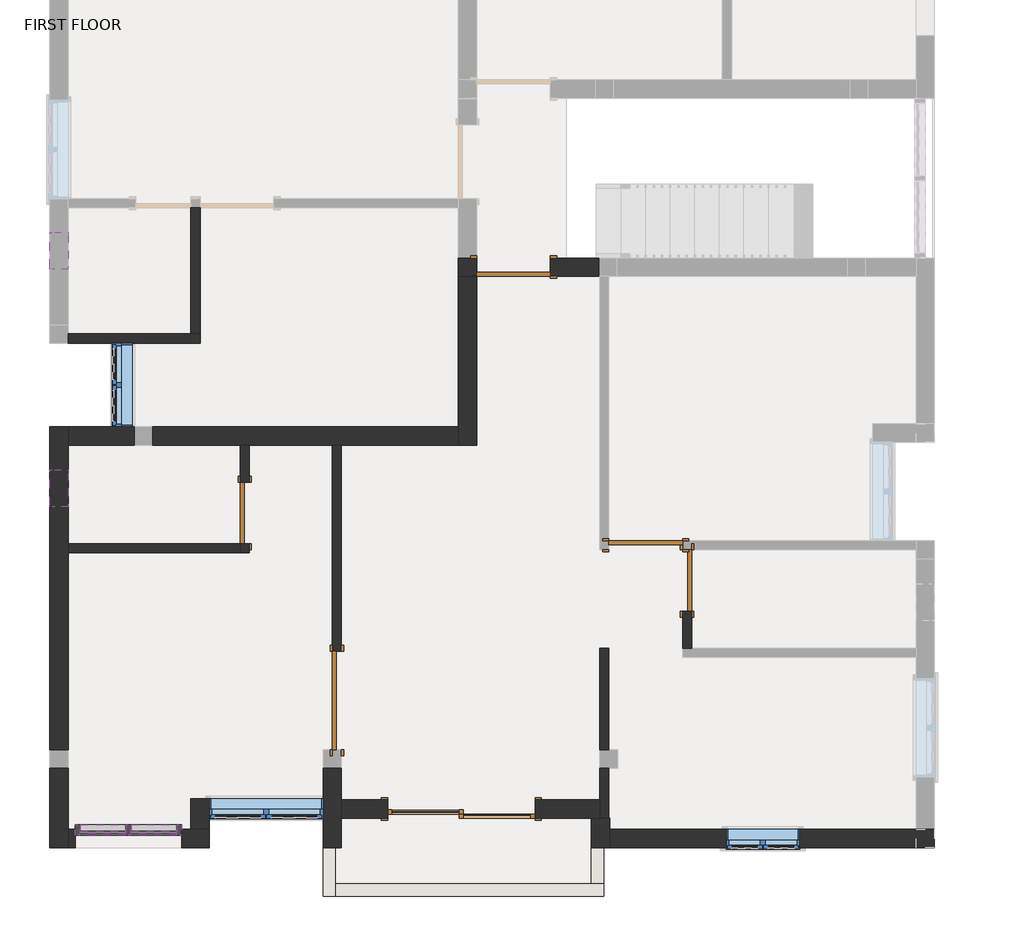
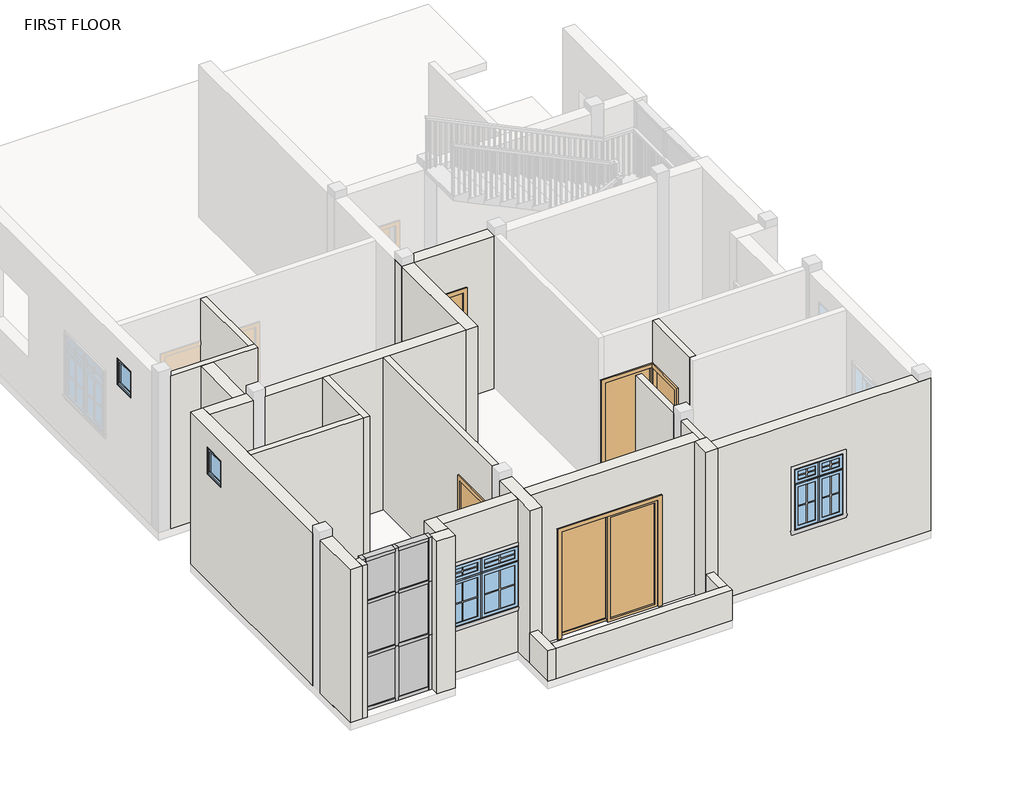
# One storey, part 1 of 6: 25 walls, 17 members, 6 doors, 6 plates, 5 windows.
"""IFC4 building model written with IfcOpenShell, lengths in millimetres."""

from ifc_helpers import new_model, si_unit, frame, origin, place, context, project, spatial, polyline, outline, extrude, faceted_brep, transform, mapped, element, save
from components import door_d4d75d1e, door_78caadf7, single_flush_3_x7_0ca8825f, single_flush_3_x7_305aa2a5, single_flush_4_x7_9343de66, member_6f432376, member_6103f85b, member_e80433b6, member_a715cb85, member_69c8e218, member_c4de40ee, member_049a2e78, member_5cd4c5ac, system_panel_glazed_fbef02e7, system_panel_glazed_b4a8312c, window_abb441dd, window_35f3c129, window_casement_double_awning_double_3_x4_7dc4ce09, window_c5cb33f6

model = new_model("IFC4")

# Units and contexts
model_context = context("Model", 3, world=origin())
ifc_project = project(units=[si_unit("LENGTHUNIT", "METRE", prefix="MILLI")], contexts=[model_context])

# Site, building, storey
site = spatial("IfcSite", under=ifc_project)
building = spatial("IfcBuilding", under=site)
storey = spatial("IfcBuildingStorey", under=building, Name="FIRST FLOOR", Elevation=3200.4)

# Doors
placement = place(None, origin())
door_shape = door_d4d75d1e(model_context)
element("IfcDoor", 1, ObjectType="Door-Double-Sliding : 72\" x 84\"", at=placement, inside=storey, context=model_context, shape_type="MappedRepresentation", body=[
    mapped(door_shape, transform((-1663.0865981, -7209.8212413, 3200.4), x_axis=(-1.0, 0.0, 0.0), y_axis=(0.0, -1.0, 0.0), z_axis=(0.0, 0.0, 1.0))),
])
door_2_shape = door_78caadf7(model_context)
element("IfcDoor", 2, ObjectType="Single-Flush : 2'6\"X7'", at=placement, inside=storey, context=model_context, shape_type="MappedRepresentation", body=[
    mapped(door_2_shape, transform((-4349.1365981, -3666.5212413, 3200.4), x_axis=(0.0, -1.0, 0.0), y_axis=(1.0, 0.0, 0.0), z_axis=(0.0, 0.0, 1.0))),
])
element("IfcDoor", 3, ObjectType="Single-Flush : 2'6\"X7'", at=placement, inside=storey, context=model_context, shape_type="MappedRepresentation", body=[
    mapped(door_2_shape, transform((1137.2634019, -4504.7212413, 3200.4), x_axis=(0.0, 1.0, 0.0), y_axis=(-1.0, 0.0, 0.0), z_axis=(0.0, 0.0, 1.0))),
])
single_flush_3_x7_shape = single_flush_3_x7_0ca8825f(model_context)
element("IfcDoor", 4, ObjectType="Single-Flush : 3'X7'", at=placement, inside=storey, context=model_context, shape_type="MappedRepresentation", body=[
    mapped(single_flush_3_x7_shape, transform((-1015.3865981, -618.5212413, 3200.4), x_axis=(-1.0, 0.0, 0.0), y_axis=(0.0, -1.0, 0.0), z_axis=(0.0, 0.0, 1.0))),
])
single_flush_3_x7_2_shape = single_flush_3_x7_305aa2a5(model_context)
element("IfcDoor", 5, ObjectType="Single-Flush : 3'X7'", at=placement, inside=storey, context=model_context, shape_type="MappedRepresentation", body=[
    mapped(single_flush_3_x7_2_shape, transform((622.9134019, -4066.5712413, 3200.4), x_axis=(-1.0, 0.0, 0.0), y_axis=(0.0, -1.0, 0.0), z_axis=(0.0, 0.0, 1.0))),
])
single_flush_4_x7_shape = single_flush_4_x7_9343de66(model_context)
element("IfcDoor", 6, ObjectType="Single-Flush : 4'X7'", at=placement, inside=storey, context=model_context, shape_type="MappedRepresentation", body=[
    mapped(single_flush_4_x7_shape, transform((-3206.1365981, -5990.6212413, 3200.4), x_axis=(0.0, -1.0, 0.0), y_axis=(1.0, 0.0, 0.0), z_axis=(0.0, 0.0, 1.0))),
])

# Members
member_shape = member_6f432376(model_context)
element("IfcMember", 7, ObjectType="Rectangular Mullion : 2.5\" x 5\" rectangular", at=placement, inside=storey, context=model_context, shape_type="MappedRepresentation", body=[
    mapped(member_shape, transform((-5193.6865981, -7597.1712413, 6248.4), x_axis=(0.0, 0.0, 1.0), y_axis=(0.0, -1.0, 0.0), z_axis=(1.0, 0.0, 0.0))),
])
element("IfcMember", 8, ObjectType="Rectangular Mullion : 2.5\" x 5\" rectangular", at=placement, inside=storey, context=model_context, shape_type="MappedRepresentation", body=[
    mapped(member_shape, transform((-5822.3365981, -7597.1712413, 6248.4), x_axis=(0.0, 0.0, 1.0), y_axis=(0.0, -1.0, 0.0), z_axis=(1.0, 0.0, 0.0))),
])
element("IfcMember", 9, ObjectType="Rectangular Mullion : 2.5\" x 5\" rectangular", at=placement, inside=storey, context=model_context, shape_type="MappedRepresentation", body=[
    mapped(member_shape, transform((-6387.4865981, -7597.1712413, 3200.4), x_axis=(0.0, 0.0, -1.0), y_axis=(0.0, -1.0, 0.0), z_axis=(-1.0, 0.0, 0.0))),
])
element("IfcMember", 10, ObjectType="Rectangular Mullion : 2.5\" x 5\" rectangular", at=placement, inside=storey, context=model_context, shape_type="MappedRepresentation", body=[
    mapped(member_shape, transform((-5758.8365981, -7597.1712413, 3200.4), x_axis=(0.0, 0.0, -1.0), y_axis=(0.0, -1.0, 0.0), z_axis=(-1.0, 0.0, 0.0))),
])
member_2_shape = member_6103f85b(model_context)
element("IfcMember", 11, ObjectType="Rectangular Mullion : 2.5\" x 5\" rectangular", at=placement, inside=storey, context=model_context, shape_type="MappedRepresentation", body=[
    mapped(member_2_shape, transform((-5822.3365981, -7597.1712413, 4298.95), x_axis=(0.0, 0.0, 1.0), y_axis=(0.0, -1.0, 0.0), z_axis=(1.0, 0.0, 0.0))),
])
element("IfcMember", 12, ObjectType="Rectangular Mullion : 2.5\" x 5\" rectangular", at=placement, inside=storey, context=model_context, shape_type="MappedRepresentation", body=[
    mapped(member_2_shape, transform((-5822.3365981, -7597.1712413, 5365.75), x_axis=(0.0, 0.0, 1.0), y_axis=(0.0, -1.0, 0.0), z_axis=(1.0, 0.0, 0.0))),
])
element("IfcMember", 13, ObjectType="Rectangular Mullion : 2.5\" x 5\" rectangular", at=placement, inside=storey, context=model_context, shape_type="MappedRepresentation", body=[
    mapped(member_2_shape, transform((-5193.6865981, -7597.1712413, 4298.95), x_axis=(0.0, 0.0, 1.0), y_axis=(0.0, -1.0, 0.0), z_axis=(1.0, 0.0, 0.0))),
])
element("IfcMember", 14, ObjectType="Rectangular Mullion : 2.5\" x 5\" rectangular", at=placement, inside=storey, context=model_context, shape_type="MappedRepresentation", body=[
    mapped(member_2_shape, transform((-5193.6865981, -7597.1712413, 5365.75), x_axis=(0.0, 0.0, 1.0), y_axis=(0.0, -1.0, 0.0), z_axis=(1.0, 0.0, 0.0))),
])
member_3_shape = member_e80433b6(model_context)
element("IfcMember", 15, ObjectType="Rectangular Mullion : 2.5\" x 5\" rectangular", at=placement, inside=storey, context=model_context, shape_type="MappedRepresentation", body=[
    mapped(member_3_shape, transform((-5790.5865981, -7597.1712413, 3200.4), x_axis=(1.0, 0.0, 0.0), y_axis=(0.0, -1.0, 0.0), z_axis=(0.0, 0.0, -1.0))),
])
member_4_shape = member_a715cb85(model_context)
element("IfcMember", 16, ObjectType="Rectangular Mullion : 2.5\" x 5\" rectangular", at=placement, inside=storey, context=model_context, shape_type="MappedRepresentation", body=[
    mapped(member_4_shape, transform((-5790.5865981, -7597.1712413, 4298.95), x_axis=(1.0, 0.0, 0.0), y_axis=(0.0, -1.0, 0.0), z_axis=(0.0, 0.0, -1.0))),
])
member_5_shape = member_69c8e218(model_context)
element("IfcMember", 17, ObjectType="Rectangular Mullion : 2.5\" x 5\" rectangular", at=placement, inside=storey, context=model_context, shape_type="MappedRepresentation", body=[
    mapped(member_5_shape, transform((-5130.1865981, -7597.1712413, 3200.4), x_axis=(1.0, 0.0, 0.0), y_axis=(0.0, -1.0, 0.0), z_axis=(0.0, 0.0, -1.0))),
])
member_6_shape = member_c4de40ee(model_context)
element("IfcMember", 18, ObjectType="Rectangular Mullion : 2.5\" x 5\" rectangular", at=placement, inside=storey, context=model_context, shape_type="MappedRepresentation", body=[
    mapped(member_6_shape, transform((-5130.1865981, -7597.1712413, 4298.95), x_axis=(1.0, 0.0, 0.0), y_axis=(0.0, -1.0, 0.0), z_axis=(0.0, 0.0, -1.0))),
])
element("IfcMember", 19, ObjectType="Rectangular Mullion : 2.5\" x 5\" rectangular", at=placement, inside=storey, context=model_context, shape_type="MappedRepresentation", body=[
    mapped(member_5_shape, transform((-6450.9865981, -7597.1712413, 4298.95), x_axis=(-1.0, 0.0, 0.0), y_axis=(0.0, -1.0, 0.0), z_axis=(0.0, 0.0, 1.0))),
])
element("IfcMember", 20, ObjectType="Rectangular Mullion : 2.5\" x 5\" rectangular", at=placement, inside=storey, context=model_context, shape_type="MappedRepresentation", body=[
    mapped(member_6_shape, transform((-6450.9865981, -7597.1712413, 5365.75), x_axis=(-1.0, 0.0, 0.0), y_axis=(0.0, -1.0, 0.0), z_axis=(0.0, 0.0, 1.0))),
])
member_7_shape = member_049a2e78(model_context)
element("IfcMember", 21, ObjectType="Rectangular Mullion : 2.5\" x 5\" rectangular", at=placement, inside=storey, context=model_context, shape_type="MappedRepresentation", body=[
    mapped(member_7_shape, transform((-5790.5865981, -7597.1712413, 5365.75), x_axis=(1.0, 0.0, 0.0), y_axis=(0.0, -1.0, 0.0), z_axis=(0.0, 0.0, -1.0))),
])
member_8_shape = member_5cd4c5ac(model_context)
element("IfcMember", 22, ObjectType="Rectangular Mullion : 2.5\" x 5\" rectangular", at=placement, inside=storey, context=model_context, shape_type="MappedRepresentation", body=[
    mapped(member_8_shape, transform((-5130.1865981, -7597.1712413, 5365.75), x_axis=(1.0, 0.0, 0.0), y_axis=(0.0, -1.0, 0.0), z_axis=(0.0, 0.0, -1.0))),
])
element("IfcMember", 23, ObjectType="Rectangular Mullion : 2.5\" x 5\" rectangular", at=placement, inside=storey, context=model_context, shape_type="MappedRepresentation", body=[
    mapped(member_8_shape, transform((-6450.9865981, -7597.1712413, 6248.4), x_axis=(-1.0, 0.0, 0.0), y_axis=(0.0, -1.0, 0.0), z_axis=(0.0, 0.0, 1.0))),
])

# Plates
system_panel_glazed_shape = system_panel_glazed_fbef02e7(model_context)
element("IfcPlate", 24, ObjectType="System Panel : Glazed", at=placement, inside=storey, context=model_context, shape_type="MappedRepresentation", body=[
    mapped(system_panel_glazed_shape, transform((-6104.9115981, -7597.1712413, 3263.9), x_axis=(1.0, 0.0, 0.0), y_axis=(0.0, 1.0, 0.0), z_axis=(0.0, 0.0, 1.0))),
])
element("IfcPlate", 25, ObjectType="System Panel : Glazed", at=placement, inside=storey, context=model_context, shape_type="MappedRepresentation", body=[
    mapped(system_panel_glazed_shape, transform((-6104.9115981, -7597.1712413, 4330.7), x_axis=(1.0, 0.0, 0.0), y_axis=(0.0, 1.0, 0.0), z_axis=(0.0, 0.0, 1.0))),
])
element("IfcPlate", 26, ObjectType="System Panel : Glazed", at=placement, inside=storey, context=model_context, shape_type="MappedRepresentation", body=[
    mapped(system_panel_glazed_shape, transform((-5476.2615981, -7597.1712413, 3263.9), x_axis=(1.0, 0.0, 0.0), y_axis=(0.0, 1.0, 0.0), z_axis=(0.0, 0.0, 1.0))),
])
element("IfcPlate", 27, ObjectType="System Panel : Glazed", at=placement, inside=storey, context=model_context, shape_type="MappedRepresentation", body=[
    mapped(system_panel_glazed_shape, transform((-5476.2615981, -7597.1712413, 4330.7), x_axis=(1.0, 0.0, 0.0), y_axis=(0.0, 1.0, 0.0), z_axis=(0.0, 0.0, 1.0))),
])
system_panel_glazed_2_shape = system_panel_glazed_b4a8312c(model_context)
element("IfcPlate", 28, ObjectType="System Panel : Glazed", at=placement, inside=storey, context=model_context, shape_type="MappedRepresentation", body=[
    mapped(system_panel_glazed_2_shape, transform((-6104.9115981, -7597.1712413, 5397.5), x_axis=(1.0, 0.0, 0.0), y_axis=(0.0, 1.0, 0.0), z_axis=(0.0, 0.0, 1.0))),
])
element("IfcPlate", 29, ObjectType="System Panel : Glazed", at=placement, inside=storey, context=model_context, shape_type="MappedRepresentation", body=[
    mapped(system_panel_glazed_2_shape, transform((-5476.2615981, -7597.1712413, 5397.5), x_axis=(1.0, 0.0, 0.0), y_axis=(0.0, 1.0, 0.0), z_axis=(0.0, 0.0, 1.0))),
])

# Walls
element("IfcWall", 30, ObjectType="4.5\"", at=placement, inside=storey, context=model_context, shape_type="Brep", body=[
    faceted_brep([(-6539.8865981, -1558.3212413, 3200.4), (-5974.2886947, -1558.3212413, 3200.4), (-5745.6886947, -1558.3212413, 3200.4), (-4901.5865981, -1558.3212413, 3200.4), (-4901.5865981, -1558.3212413, 6248.4), (-5745.6886947, -1558.3212413, 6248.4), (-5974.2886947, -1558.3212413, 6248.4), (-6539.8865981, -1558.3212413, 6248.4), (-6539.8865981, -1444.0212413, 3200.4), (-6539.8865981, -1444.0212413, 6248.4), (-5015.8865981, -1444.0212413, 6248.4), (-4901.5865981, -1444.0212413, 6248.4), (-4901.5865981, -1444.0212413, 3200.4), (-5015.8865981, -1444.0212413, 3200.4)], [[[0, 1, 2, 3, 4, 5, 6, 7]], [[8, 9, 10, 11, 12, 13]], [[3, 2, 1, 0, 8, 13, 12]], [[7, 6, 5, 4, 11, 10, 9]], [[0, 7, 9, 8]], [[4, 3, 12, 11]]]),
])
element("IfcWall", 31, ObjectType="4.5\"", at=placement, inside=storey, context=model_context, shape_type="SweptSolid", body=[
    extrude(outline(polyline([(-4901.5865981, 118.0787587), (-4901.5865981, -1444.0212413), (-5015.8865981, -1444.0212413), (-5015.8865981, 118.0787587), (-4901.5865981, 118.0787587)])), frame((0.0, 0.0, 3200.4), z_axis=(0.0, 0.0, 1.0), x_axis=(1.0, 0.0, 0.0)), (0.0, 0.0, 1.0), 3048.0),
])
element("IfcWall", 32, ObjectType="4.5\"", at=placement, inside=storey, context=model_context, shape_type="Brep", body=[
    faceted_brep([(-4406.2865981, -4047.5212413, 5334.0), (-4406.2865981, -4047.5212413, 3200.4), (-4406.2865981, -4161.8212413, 3200.4), (-4406.2865981, -4161.8212413, 6248.4), (-4406.2865981, -4047.5212413, 6248.4), (-4406.2865981, -2828.3212413, 6248.4), (-4406.2865981, -2828.3212413, 3200.4), (-4406.2865981, -3285.5212413, 3200.4), (-4406.2865981, -3285.5212413, 5334.0), (-4291.9865981, -4161.8212413, 3200.4), (-4291.9865981, -4047.5212413, 3200.4), (-4291.9865981, -4047.5212413, 5334.0), (-4291.9865981, -3285.5212413, 5334.0), (-4291.9865981, -3285.5212413, 3200.4), (-4291.9865981, -2828.3212413, 3200.4), (-4291.9865981, -2828.3212413, 6248.4), (-4291.9865981, -4161.8212413, 6248.4)], [[[0, 1, 2, 3, 4, 5, 6, 7, 8]], [[9, 10, 11, 12, 13, 14, 15, 16]], [[7, 6, 14, 13]], [[2, 1, 10, 9]], [[5, 4, 3, 16, 15]], [[6, 5, 15, 14]], [[3, 2, 9, 16]], [[11, 10, 1, 0]], [[12, 11, 0, 8]], [[13, 12, 8, 7]]]),
])
element("IfcWall", 33, ObjectType="4.5\"", at=placement, inside=storey, context=model_context, shape_type="SweptSolid", body=[
    extrude(outline(polyline([(-6539.8865981, -4047.5212413), (-4406.2865981, -4047.5212413), (-4406.2865981, -4161.8212413), (-6539.8865981, -4161.8212413), (-6539.8865981, -4047.5212413)])), frame((0.0, 0.0, 3200.4), z_axis=(0.0, 0.0, 1.0), x_axis=(1.0, 0.0, 0.0)), (0.0, 0.0, 1.0), 3048.0),
])
element("IfcWall", 34, ObjectType="4.5\"", at=placement, inside=storey, context=model_context, shape_type="SweptSolid", body=[
    extrude(outline(polyline([(-6600.2212413, 6248.4), (-2828.3212413, 6248.4), (-2828.3212413, 3200.4), (-5381.0212413, 3200.4), (-5381.0212413, 5334.0), (-6600.2212413, 5334.0), (-6600.2212413, 6248.4)])), frame((-3263.2865981, 0.0, 0.0), z_axis=(1.0, 0.0, 0.0), x_axis=(0.0, 1.0, 0.0)), (0.0, 0.0, 1.0), 114.3),
])
element("IfcWall", 35, ObjectType="4.5\"", at=placement, inside=storey, context=model_context, shape_type="SweptSolid", body=[
    extrude(outline(polyline([(-5342.9212413, 6248.4), (-4123.7212413, 6248.4), (-4123.7212413, 5334.0), (-4885.7212413, 5334.0), (-4885.7212413, 3200.4), (-5342.9212413, 3200.4), (-5342.9212413, 6248.4)])), frame((1080.1134019, 0.0, 0.0), z_axis=(1.0, 0.0, 0.0), x_axis=(0.0, 1.0, 0.0)), (0.0, 0.0, 1.0), 114.3),
])
element("IfcWall", 36, ObjectType="4.5\"", at=placement, inside=storey, context=model_context, shape_type="SweptSolid", body=[
    extrude(outline(polyline([(51.4134019, -6601.1424416), (51.4134019, -5342.9212413), (165.7134019, -5342.9212413), (165.7134019, -6601.1424416), (51.4134019, -6601.1424416)])), frame((0.0, 0.0, 3200.4), z_axis=(0.0, 0.0, 1.0), x_axis=(1.0, 0.0, 0.0)), (0.0, 0.0, 1.0), 3048.0),
])
element("IfcWall", 37, ObjectType="4.5\"", at=placement, inside=storey, context=model_context, shape_type="Brep", body=[
    faceted_brep([(51.4134019, -6829.7424416, 3200.4), (51.4134019, -7222.5212413, 3200.4), (51.4134019, -7451.1212413, 3200.4), (51.4134019, -7451.1212413, 6248.4), (51.4134019, -7222.5212413, 6248.4), (51.4134019, -6829.7424416, 6248.4), (165.7134019, -6829.7424416, 3200.4), (165.7134019, -6829.7424416, 6248.4), (165.7134019, -7451.1212413, 6248.4), (165.7134019, -7451.1212413, 3200.4)], [[[0, 1, 2, 3, 4, 5]], [[6, 7, 8, 9]], [[2, 1, 0, 6, 9]], [[5, 4, 3, 8, 7]], [[0, 5, 7, 6]], [[3, 2, 9, 8]]]),
])
element("IfcWall", 38, ObjectType="6\"", at=placement, inside=storey, context=model_context, shape_type="Brep", body=[
    faceted_brep([(-3377.5865981, -7819.4212413, 3200.4), (-3377.5865981, -8416.3212413, 3200.4), (-3377.5865981, -8416.3212413, 3810.0), (-3377.5865981, -7819.4212413, 3810.0), (-3225.1865981, -7819.4212413, 3200.4), (-3225.1865981, -7819.4212413, 3810.0), (-3225.1865981, -8263.9212413, 3810.0), (-3225.1865981, -8416.3212413, 3810.0), (-3225.1865981, -8416.3212413, 3200.4), (-3225.1865981, -8263.9212413, 3200.4)], [[[0, 1, 2, 3]], [[4, 5, 6, 7, 8, 9]], [[1, 0, 4, 9, 8]], [[3, 2, 7, 6, 5]], [[0, 3, 5, 4]], [[2, 1, 8, 7]]]),
])
element("IfcWall", 39, ObjectType="6\"", at=placement, inside=storey, context=model_context, shape_type="Brep", body=[
    faceted_brep([(-3225.1865981, -8416.3212413, 3200.4), (102.2134019, -8416.3212413, 3200.4), (102.2134019, -8416.3212413, 3810.0), (-3225.1865981, -8416.3212413, 3810.0), (-3225.1865981, -8263.9212413, 3200.4), (-3225.1865981, -8263.9212413, 3810.0), (-50.1865981, -8263.9212413, 3810.0), (102.2134019, -8263.9212413, 3810.0), (102.2134019, -8263.9212413, 3200.4), (-50.1865981, -8263.9212413, 3200.4)], [[[0, 1, 2, 3]], [[4, 5, 6, 7, 8, 9]], [[1, 0, 4, 9, 8]], [[3, 2, 7, 6, 5]], [[0, 3, 5, 4]], [[2, 1, 8, 7]]]),
])
element("IfcWall", 40, ObjectType="6\"", at=placement, inside=storey, context=model_context, shape_type="SweptSolid", body=[
    extrude(outline(polyline([(102.2134019, -7819.4212413), (102.2134019, -8263.9212413), (-50.1865981, -8263.9212413), (-50.1865981, -7819.4212413), (102.2134019, -7819.4212413)])), frame((0.0, 0.0, 3200.4), z_axis=(0.0, 0.0, 1.0), x_axis=(1.0, 0.0, 0.0)), (0.0, 0.0, 1.0), 609.6),
])
element("IfcWall", 41, ObjectType="9\"", at=placement, inside=storey, context=model_context, shape_type="Brep", body=[
    faceted_brep([(-6768.4865981, -2599.7212413, 3200.4), (-6768.4865981, -6601.1424416, 3200.4), (-6768.4865981, -6601.1424416, 6248.4), (-6768.4865981, -2599.7212413, 6248.4), (-6768.4865981, -3133.1212413, 5867.4), (-6768.4865981, -3590.3212413, 5867.4), (-6768.4865981, -3590.3212413, 5334.0), (-6768.4865981, -3133.1212413, 5334.0), (-6539.8865981, -2599.7212413, 3200.4), (-6539.8865981, -2599.7212413, 6248.4), (-6539.8865981, -2828.3212413, 6248.4), (-6539.8865981, -4047.5212413, 6248.4), (-6539.8865981, -4161.8212413, 6248.4), (-6539.8865981, -6601.1424416, 6248.4), (-6539.8865981, -6601.1424416, 3200.4), (-6539.8865981, -4161.8212413, 3200.4), (-6539.8865981, -4047.5212413, 3200.4), (-6539.8865981, -2828.3212413, 3200.4), (-6539.8865981, -3133.1212413, 5867.4), (-6539.8865981, -3133.1212413, 5334.0), (-6539.8865981, -3590.3212413, 5334.0), (-6539.8865981, -3590.3212413, 5867.4)], [[[0, 1, 2, 3], [4, 5, 6, 7]], [[8, 9, 10, 11, 12, 13, 14, 15, 16, 17], [18, 19, 20, 21]], [[1, 0, 8, 17, 16, 15, 14]], [[2, 1, 14, 13]], [[3, 2, 13, 12, 11, 10, 9]], [[0, 3, 9, 8]], [[19, 18, 4, 7]], [[20, 19, 7, 6]], [[21, 20, 6, 5]], [[18, 21, 5, 4]]]),
])
element("IfcWall", 42, ObjectType="9\"", at=placement, inside=storey, context=model_context, shape_type="Brep", body=[
    faceted_brep([(-6768.4865981, -6829.7424416, 3200.4), (-6768.4865981, -7819.4212413, 3200.4), (-6768.4865981, -7819.4212413, 6248.4), (-6768.4865981, -6829.7424416, 6248.4), (-6539.8865981, -6829.7424416, 3200.4), (-6539.8865981, -6829.7424416, 6248.4), (-6539.8865981, -7590.8212413, 6248.4), (-6539.8865981, -7819.4212413, 6248.4), (-6539.8865981, -7819.4212413, 3200.4), (-6539.8865981, -7590.8212413, 3200.4)], [[[0, 1, 2, 3]], [[4, 5, 6, 7, 8, 9]], [[1, 0, 4, 9, 8]], [[3, 2, 7, 6, 5]], [[0, 3, 5, 4]], [[2, 1, 8, 7]]]),
])
element("IfcWall", 43, ObjectType="9\"", at=placement, inside=storey, context=model_context, shape_type="Brep", body=[
    faceted_brep([(-6539.8865981, -7819.4212413, 6248.4), (-6539.8865981, -7819.4212413, 3200.4), (-6450.9865981, -7819.4212413, 3200.4), (-6450.9865981, -7819.4212413, 6248.4), (-6539.8865981, -7590.8212413, 3200.4), (-6539.8865981, -7590.8212413, 6248.4), (-6450.9865981, -7590.8212413, 6248.4), (-6450.9865981, -7590.8212413, 3200.4)], [[[0, 1, 2, 3]], [[4, 5, 6, 7]], [[1, 4, 7, 2]], [[5, 0, 3, 6]], [[1, 0, 5, 4]], [[3, 2, 7, 6]]]),
    faceted_brep([(-4787.2865981, -7819.4212413, 3200.4), (-4787.2865981, -7819.4212413, 6248.4), (-5130.1865981, -7819.4212413, 6248.4), (-5130.1865981, -7819.4212413, 3200.4), (-4787.2865981, -7590.8212413, 6248.4), (-4787.2865981, -7590.8212413, 3200.4), (-5015.8865981, -7590.8212413, 3200.4), (-5130.1865981, -7590.8212413, 3200.4), (-5130.1865981, -7590.8212413, 6248.4), (-5015.8865981, -7590.8212413, 6248.4)], [[[0, 1, 2, 3]], [[4, 5, 6, 7, 8, 9]], [[5, 0, 3, 7, 6]], [[1, 4, 9, 8, 2]], [[1, 0, 5, 4]], [[3, 2, 8, 7]]]),
])
element("IfcWall", 44, ObjectType="9\"", at=placement, inside=storey, context=model_context, shape_type="Brep", body=[
    faceted_brep([(-4787.2865981, -7590.8212413, 3200.4), (-4787.2865981, -7438.4212413, 3200.4), (-4787.2865981, -7209.8212413, 3200.4), (-4787.2865981, -7209.8212413, 4114.8), (-4787.2865981, -7209.8212413, 5334.0), (-4787.2865981, -7209.8212413, 6248.4), (-4787.2865981, -7438.4212413, 6248.4), (-4787.2865981, -7590.8212413, 6248.4), (-5015.8865981, -7590.8212413, 3200.4), (-5015.8865981, -7590.8212413, 6248.4), (-5015.8865981, -7209.8212413, 6248.4), (-5015.8865981, -7209.8212413, 3200.4)], [[[0, 1, 2, 3, 4, 5, 6, 7]], [[8, 9, 10, 11]], [[2, 1, 0, 8, 11]], [[7, 6, 5, 10, 9]], [[0, 7, 9, 8]], [[5, 4, 3, 2, 11, 10]]]),
])
element("IfcWall", 45, ObjectType="9\"", at=placement, inside=storey, context=model_context, shape_type="SweptSolid", body=[
    extrude(outline(polyline([(-3377.5865981, -7438.4212413), (-4787.2865981, -7438.4212413), (-4787.2865981, -7209.8212413), (-3377.5865981, -7209.8212413), (-3377.5865981, -7438.4212413)])), frame((0.0, 0.0, 3200.4), z_axis=(0.0, 0.0, 1.0), x_axis=(1.0, 0.0, 0.0)), (0.0, 0.0, 1.0), 914.4),
    extrude(outline(polyline([(-3377.5865981, -7438.4212413), (-4787.2865981, -7438.4212413), (-4787.2865981, -7209.8212413), (-3377.5865981, -7209.8212413), (-3377.5865981, -7438.4212413)])), frame((0.0, 0.0, 5334.0), z_axis=(0.0, 0.0, 1.0), x_axis=(1.0, 0.0, 0.0)), (0.0, 0.0, 1.0), 914.4),
])
element("IfcWall", 46, ObjectType="9\"", at=placement, inside=storey, context=model_context, shape_type="Brep", body=[
    faceted_brep([(-3377.5865981, -6828.8212413, 3200.4), (-3377.5865981, -7209.8212413, 3200.4), (-3377.5865981, -7438.4212413, 3200.4), (-3377.5865981, -7819.4212413, 3200.4), (-3377.5865981, -7819.4212413, 3810.0), (-3377.5865981, -7819.4212413, 6248.4), (-3377.5865981, -7438.4212413, 6248.4), (-3377.5865981, -7209.8212413, 6248.4), (-3377.5865981, -6828.8212413, 6248.4), (-3148.9865981, -6828.8212413, 3200.4), (-3148.9865981, -6828.8212413, 6248.4), (-3148.9865981, -7222.5212413, 6248.4), (-3148.9865981, -7451.1212413, 6248.4), (-3148.9865981, -7819.4212413, 6248.4), (-3148.9865981, -7819.4212413, 3200.4), (-3148.9865981, -7451.1212413, 3200.4), (-3148.9865981, -7222.5212413, 3200.4), (-3225.1865981, -7819.4212413, 3200.4)], [[[0, 1, 2, 3, 4, 5, 6, 7, 8]], [[9, 10, 11, 12, 13, 14, 15, 16]], [[3, 2, 1, 0, 9, 16, 15, 14, 17]], [[5, 4, 3, 17, 14, 13]], [[8, 7, 6, 5, 13, 12, 11, 10]], [[0, 8, 10, 9]]]),
])
element("IfcWall", 47, ObjectType="9\"", at=placement, inside=storey, context=model_context, shape_type="Brep", body=[
    faceted_brep([(-2577.4865981, -7222.5212413, 5334.0), (-2577.4865981, -7222.5212413, 3200.4), (-3148.9865981, -7222.5212413, 3200.4), (-3148.9865981, -7222.5212413, 6248.4), (51.4134019, -7222.5212413, 6248.4), (51.4134019, -7222.5212413, 3200.4), (-748.6865981, -7222.5212413, 3200.4), (-748.6865981, -7222.5212413, 5334.0), (-3148.9865981, -7451.1212413, 3200.4), (-2577.4865981, -7451.1212413, 3200.4), (-2577.4865981, -7451.1212413, 5334.0), (-748.6865981, -7451.1212413, 5334.0), (-748.6865981, -7451.1212413, 3200.4), (-50.1865981, -7451.1212413, 3200.4), (51.4134019, -7451.1212413, 3200.4), (51.4134019, -7451.1212413, 6248.4), (-50.1865981, -7451.1212413, 6248.4), (-3148.9865981, -7451.1212413, 6248.4)], [[[0, 1, 2, 3, 4, 5, 6, 7]], [[8, 9, 10, 11, 12, 13, 14, 15, 16, 17]], [[6, 5, 14, 13, 12]], [[2, 1, 9, 8]], [[4, 3, 17, 16, 15]], [[3, 2, 8, 17]], [[5, 4, 15, 14]], [[12, 11, 7, 6]], [[10, 9, 1, 0]], [[11, 10, 0, 7]]]),
])
element("IfcWall", 48, ObjectType="9\"", at=placement, inside=storey, context=model_context, shape_type="Brep", body=[
    faceted_brep([(-50.1865981, -7451.1212413, 3200.4), (-50.1865981, -7819.4212413, 3200.4), (-50.1865981, -7819.4212413, 3810.0), (-50.1865981, -7819.4212413, 6248.4), (-50.1865981, -7451.1212413, 6248.4), (178.4134019, -7451.1212413, 3200.4), (178.4134019, -7451.1212413, 6248.4), (178.4134019, -7590.8212413, 6248.4), (178.4134019, -7819.4212413, 6248.4), (178.4134019, -7819.4212413, 3200.4), (178.4134019, -7590.8212413, 3200.4), (51.4134019, -7451.1212413, 3200.4), (165.7134019, -7451.1212413, 3200.4), (102.2134019, -7819.4212413, 3200.4), (165.7134019, -7451.1212413, 6248.4), (51.4134019, -7451.1212413, 6248.4)], [[[0, 1, 2, 3, 4]], [[5, 6, 7, 8, 9, 10]], [[1, 0, 11, 12, 5, 10, 9, 13]], [[4, 3, 8, 7, 6, 14, 15]], [[0, 4, 15, 14, 6, 5, 12, 11]], [[1, 13, 9, 8, 3, 2]]]),
])
element("IfcWall", 49, ObjectType="9\"", at=placement, inside=storey, context=model_context, shape_type="Brep", body=[
    faceted_brep([(178.4134019, -7819.4212413, 6248.4), (178.4134019, -7819.4212413, 3200.4), (4204.3134019, -7819.4212413, 3200.4), (4204.3134019, -7819.4212413, 6248.4), (3975.7134019, -7819.4212413, 6248.4), (1619.8634019, -7819.4212413, 5334.0), (2534.2634019, -7819.4212413, 5334.0), (2534.2634019, -7819.4212413, 4114.8), (1619.8634019, -7819.4212413, 4114.8), (178.4134019, -7590.8212413, 3200.4), (178.4134019, -7590.8212413, 6248.4), (3975.7134019, -7590.8212413, 6248.4), (4204.3134019, -7590.8212413, 6248.4), (4204.3134019, -7590.8212413, 3200.4), (3975.7134019, -7590.8212413, 3200.4), (1619.8634019, -7590.8212413, 5334.0), (1619.8634019, -7590.8212413, 4114.8), (2534.2634019, -7590.8212413, 4114.8), (2534.2634019, -7590.8212413, 5334.0)], [[[0, 1, 2, 3, 4], [5, 6, 7, 8]], [[9, 10, 11, 12, 13, 14], [15, 16, 17, 18]], [[2, 1, 9, 14, 13]], [[0, 4, 3, 12, 11, 10]], [[3, 2, 13, 12]], [[0, 10, 9, 1]], [[16, 15, 5, 8]], [[17, 16, 8, 7]], [[18, 17, 7, 6]], [[15, 18, 6, 5]]]),
])
element("IfcWall", 50, ObjectType="9\"", at=placement, inside=storey, context=model_context, shape_type="Brep", body=[
    faceted_brep([(-1472.5865981, -504.2212413, 5334.0), (-1472.5865981, -504.2212413, 3200.4), (-1701.1865981, -504.2212413, 3200.4), (-1701.1865981, -504.2212413, 6248.4), (-1472.5865981, -504.2212413, 6248.4), (41.1035962, -504.2212413, 6248.4), (41.1035962, -504.2212413, 3200.4), (-558.1865981, -504.2212413, 3200.4), (-558.1865981, -504.2212413, 5334.0), (-1701.1865981, -732.8212413, 3200.4), (-1472.5865981, -732.8212413, 3200.4), (-1472.5865981, -732.8212413, 5334.0), (-558.1865981, -732.8212413, 5334.0), (-558.1865981, -732.8212413, 3200.4), (41.1035962, -732.8212413, 3200.4), (41.1035962, -732.8212413, 6248.4), (-1472.5865981, -732.8212413, 6248.4), (-1701.1865981, -732.8212413, 6248.4), (-1701.1865981, -505.1424416, 6248.4)], [[[0, 1, 2, 3, 4, 5, 6, 7, 8]], [[9, 10, 11, 12, 13, 14, 15, 16, 17]], [[7, 6, 14, 13]], [[2, 1, 10, 9]], [[5, 4, 3, 18, 17, 16, 15]], [[6, 5, 15, 14]], [[3, 2, 9, 17, 18]], [[11, 10, 1, 0]], [[12, 11, 0, 8]], [[13, 12, 8, 7]]]),
])
element("IfcWall", 51, ObjectType="9\"", at=placement, inside=storey, context=model_context, shape_type="Brep", body=[
    faceted_brep([(-1701.1865981, -733.7424416, 3200.4), (-1701.1865981, -2599.7212413, 3200.4), (-1701.1865981, -2828.3212413, 3200.4), (-1701.1865981, -2828.3212413, 6248.4), (-1701.1865981, -2599.7212413, 6248.4), (-1701.1865981, -733.7424416, 6248.4), (-1472.5865981, -733.7424416, 3200.4), (-1472.5865981, -733.7424416, 6248.4), (-1472.5865981, -2828.3212413, 6248.4), (-1472.5865981, -2828.3212413, 3200.4)], [[[0, 1, 2, 3, 4, 5]], [[6, 7, 8, 9]], [[2, 1, 0, 6, 9]], [[5, 4, 3, 8, 7]], [[0, 5, 7, 6]], [[3, 2, 9, 8]]]),
])
element("IfcWall", 52, ObjectType="9\"", at=placement, inside=storey, context=model_context, shape_type="Brep", body=[
    faceted_brep([(-1701.1865981, -2599.7212413, 3200.4), (-5488.7582398, -2599.7212413, 3200.4), (-5488.7582398, -2599.7212413, 6248.4), (-1701.1865981, -2599.7212413, 6248.4), (-1701.1865981, -2828.3212413, 3200.4), (-1701.1865981, -2828.3212413, 6248.4), (-3148.9865981, -2828.3212413, 6248.4), (-3263.2865981, -2828.3212413, 6248.4), (-4291.9865981, -2828.3212413, 6248.4), (-4406.2865981, -2828.3212413, 6248.4), (-5488.7582398, -2828.3212413, 6248.4), (-5488.7582398, -2828.3212413, 3200.4), (-4406.2865981, -2828.3212413, 3200.4), (-4291.9865981, -2828.3212413, 3200.4), (-3263.2865981, -2828.3212413, 3200.4), (-3148.9865981, -2828.3212413, 3200.4)], [[[0, 1, 2, 3]], [[4, 5, 6, 7, 8, 9, 10, 11, 12, 13, 14, 15]], [[1, 0, 4, 15, 14, 13, 12, 11]], [[2, 1, 11, 10]], [[3, 2, 10, 9, 8, 7, 6, 5]], [[0, 3, 5, 4]]]),
])
element("IfcWall", 53, ObjectType="9\"", at=placement, inside=storey, context=model_context, shape_type="Brep", body=[
    faceted_brep([(-5717.3582398, -2599.7212413, 3200.4), (-5745.6886947, -2599.7212413, 3200.4), (-5974.2886947, -2599.7212413, 3200.4), (-6539.8865981, -2599.7212413, 3200.4), (-6539.8865981, -2599.7212413, 6248.4), (-5974.2886947, -2599.7212413, 6248.4), (-5745.6886947, -2599.7212413, 6248.4), (-5717.3582398, -2599.7212413, 6248.4), (-5717.3582398, -2828.3212413, 3200.4), (-5717.3582398, -2828.3212413, 6248.4), (-6539.8865981, -2828.3212413, 6248.4), (-6539.8865981, -2828.3212413, 3200.4)], [[[0, 1, 2, 3, 4, 5, 6, 7]], [[8, 9, 10, 11]], [[3, 2, 1, 0, 8, 11]], [[7, 6, 5, 4, 10, 9]], [[0, 7, 9, 8]], [[4, 3, 11, 10]]]),
])
element("IfcWall", 54, ObjectType="9\"", at=placement, inside=storey, context=model_context, shape_type="SweptSolid", body=[
    extrude(outline(polyline([(-5974.2886947, -2599.7212413), (-5974.2886947, -1558.3212413), (-5745.6886947, -1558.3212413), (-5745.6886947, -2599.7212413), (-5974.2886947, -2599.7212413)])), frame((0.0, 0.0, 3200.4), z_axis=(0.0, 0.0, 1.0), x_axis=(1.0, 0.0, 0.0)), (0.0, 0.0, 1.0), 914.4),
    extrude(outline(polyline([(-5974.2886947, -2599.7212413), (-5974.2886947, -1558.3212413), (-5745.6886947, -1558.3212413), (-5745.6886947, -2599.7212413), (-5974.2886947, -2599.7212413)])), frame((0.0, 0.0, 5334.0), z_axis=(0.0, 0.0, 1.0), x_axis=(1.0, 0.0, 0.0)), (0.0, 0.0, 1.0), 914.4),
])

# Windows
window_shape = window_abb441dd(model_context)
element("IfcWindow", 55, ObjectType="Fixed : 1'6\"X1'9\"", at=placement, inside=storey, context=model_context, shape_type="MappedRepresentation", body=[
    mapped(window_shape, transform((-6654.1865981, -3323.6212413, 3200.4), x_axis=(0.0, 1.0, 0.0), y_axis=(-1.0, 0.0, 0.0), z_axis=(0.0, 0.0, 1.0))),
])
element("IfcWindow", 56, ObjectType="Fixed : 1'6\"X1'9\"", at=placement, inside=storey, context=model_context, shape_type="MappedRepresentation", body=[
    mapped(window_shape, transform((-6654.1865981, -377.2212413, 3200.4), x_axis=(0.0, 1.0, 0.0), y_axis=(-1.0, 0.0, 0.0), z_axis=(0.0, 0.0, 1.0))),
])
window_2_shape = window_35f3c129(model_context)
element("IfcWindow", 57, ObjectType="Window-Casement-Double-Awning-Double : 3'5\"X7'", at=placement, inside=storey, context=model_context, shape_type="MappedRepresentation", body=[
    mapped(window_2_shape, transform((-5859.9886947, -2079.0212413, 3200.4), x_axis=(0.0, 1.0, 0.0), y_axis=(-1.0, 0.0, 0.0), z_axis=(0.0, 0.0, 1.0))),
])
window_casement_double_awning_double_3_x4_shape = window_casement_double_awning_double_3_x4_7dc4ce09(model_context)
element("IfcWindow", 58, ObjectType="Window-Casement-Double-Awning-Double : 3'X4'", at=placement, inside=storey, context=model_context, shape_type="MappedRepresentation", body=[
    mapped(window_casement_double_awning_double_3_x4_shape, transform((2077.0634019, -7705.1212413, 3200.4), x_axis=(-1.0, 0.0, 0.0), y_axis=(0.0, -1.0, 0.0), z_axis=(0.0, 0.0, 1.0))),
])
window_3_shape = window_c5cb33f6(model_context)
element("IfcWindow", 59, ObjectType="Window-Casement-Double-Awning-Double : 4'7.5\"X4'", at=placement, inside=storey, context=model_context, shape_type="MappedRepresentation", body=[
    mapped(window_3_shape, transform((-4082.4365981, -7324.1212413, 3200.4), x_axis=(-1.0, 0.0, 0.0), y_axis=(0.0, -1.0, 0.0), z_axis=(0.0, 0.0, 1.0))),
])

save(model, "model.ifc")

# Revit data of these elements
# Type "Door-Double-Sliding : 72\" x 84\""
#   Type Mark = "13"
#   Construction Type Id = "opn-d45"
#   Assembly Code = "C1020"
#   Analytic Construction = "Wood frame, double glass door "
#   Thickness = 0' - 2"
#   Thermal Resistance (R) = 1.8150 (h·ft²·°F)/BTU
#   Heat Transfer Coefficient (U) = 0.5510 BTU/(h·ft²·°F)
#   Height = 7' - 0"
#   Rail Width = 0' - 2"
#   Stiles = 0' - 2"
#   Trim Projection Ext = 0' - 1"
#   Trim Projection Int = 0' - 1"
#   Trim Width = 0' - 3"
#   Width = 6' - 0"
#   Define Thermal Properties by = 1
#   Glazing = Glass
#   Panel Material = Wood - Birch - Solid Stained Light Low Gloss
#   Trim Material = Paint - Sienna
#   Visual Light Transmittance = 0
#   Solar Heat Gain Coefficient = 0
#   Function = (empty or 0)
#   Wall Closure = (empty or 0)
# Type "Single-Flush : 2'6\"X7'"
#   Type Mark = "9"
#   Construction Type Id = "MDOOR"
#   Assembly Code = "C1020"
#   Analytic Construction = "Metal"
#   Thickness = 0' - 2"
#   Heat Transfer Coefficient (U) = 0.651978 BTU/(h·ft²·°F)
#   Height = 7' - 0"
#   Trim Projection Ext = 0' - 1"
#   Trim Projection Int = 0' - 1"
#   Trim Width = 0' - 3"
#   Width = 2' - 6"
#   Define Thermal Properties by = 1
#   Door Material = Door - Panel
#   Frame Material = Door - Frame
#   Visual Light Transmittance = 0
#   Solar Heat Gain Coefficient = 0
#   Function = (empty or 0)
#   Wall Closure = (empty or 0)
# Type "Single-Flush : 3'X7'"
#   Type Mark = "8"
#   Construction Type Id = "MDOOR"
#   Assembly Code = "C1020"
#   Analytic Construction = "Metal"
#   Thickness = 0' - 2"
#   Heat Transfer Coefficient (U) = 0.651978 BTU/(h·ft²·°F)
#   Height = 7' - 0"
#   Trim Projection Ext = 0' - 1"
#   Trim Projection Int = 0' - 1"
#   Trim Width = 0' - 3"
#   Width = 3' - 0"
#   Define Thermal Properties by = 1
#   Door Material = Door - Panel
#   Frame Material = Door - Frame
#   Visual Light Transmittance = 0
#   Solar Heat Gain Coefficient = 0
#   Function = (empty or 0)
#   Wall Closure = (empty or 0)
# Type "Single-Flush : 4'X7'"
#   Type Mark = "12"
#   Construction Type Id = "MDOOR"
#   Assembly Code = "C1020"
#   Analytic Construction = "Metal"
#   Thickness = 0' - 2"
#   Heat Transfer Coefficient (U) = 0.651978 BTU/(h·ft²·°F)
#   Height = 7' - 0"
#   Trim Projection Ext = 0' - 1"
#   Trim Projection Int = 0' - 1"
#   Trim Width = 0' - 3"
#   Width = 4' - 0"
#   Define Thermal Properties by = 1
#   Door Material = Door - Panel
#   Frame Material = Door - Frame
#   Visual Light Transmittance = 0
#   Solar Heat Gain Coefficient = 0
#   Function = (empty or 0)
#   Wall Closure = (empty or 0)
# Type "Rectangular Mullion : 2.5\" x 5\" rectangular"
#   built-in parameter 1007304 = 0.416667 (stored number, unit not read)
#   built-in parameter 1007301 = 0.104167 (stored number, unit not read)
#   built-in parameter 1007300 = 0.104167 (stored number, unit not read)
# Type "System Panel : Glazed"
#   Construction Type Id = "GSP4R"
#   Analytic Construction = "1/8 in Pilkington single glazing"
#   Visual Light Transmittance = 0.9
#   Solar Heat Gain Coefficient = 0.86
#   Heat Transfer Coefficient (U) = 1.18115 BTU/(h·ft²·°F)
#   Define Thermal Properties by = 1
# Type "4.5\""
#   Assembly Code = "B2010"
#   Layers, outside or top first: 0' - 4 1/2" no material (function 1)
# Type "6\""
#   Assembly Code = "B2010"
#   Layers, outside or top first: 0' - 6" "wood 1" (function 1)
# Type "9\""
#   Assembly Code = "B2010"
#   Layers, outside or top first: 0' - 9" "wall" (function 1)
# Type "Fixed : 1'6\"X1'9\""
#   Type Mark = "24"
#   Construction Type Id = "GSP4R"
#   Assembly Code = "B2020100"
#   Analytic Construction = "1/8 in Pilkington single glazing"
#   Visual Light Transmittance = 0.9
#   Solar Heat Gain Coefficient = 0.78
#   Heat Transfer Coefficient (U) = 0.6496 BTU/(h·ft²·°F)
#   Height = 1' - 9"
#   Default Sill Height = 7' - 0"
#   Width = 1' - 6"
#   Window Inset = 0' - 0 3/4"
#   Define Thermal Properties by = 1
#   Glass Pane Material = Glass
#   Sash Material = Sash
#   Wall Closure = (empty or 0)
# Type "Window-Casement-Double-Awning-Double : 3'5\"X7'"
#   Type Mark = "22"
#   Fire Rating = "0.5h"
#   Assembly Code = "B2020100"
#   Analytic Construction = "Double glazing - domestic"
#   Window Inset [instance default] = 0' - 0"
#   Wall Thickness [instance default] = 0' - 6"
#   Interior Wall Closure [instance default] = 0' - 2 1/4"
#   Half Width = 1' - 8 1/2"
#   Visual Light Transmittance = 0.81
#   Transom Height = 1' - 0"
#   Thermal Resistance (R) = 1.8146 (h·ft²·°F)/BTU
#   Solar Heat Gain Coefficient = 0.76
#   Rough Width = 3' - 5 1/2"
#   Rough Height = 4' - 0 1/2"
#   Open Window Height = 3' - 0"
#   Frame Extension [instance default] = 0' - 0 1/4"
#   Height = 4' - 0"
#   Heat Transfer Coefficient (U) = 0.5511 BTU/(h·ft²·°F)
#   Exterior Wall Closure [instance default] = 0' - 1 1/4"
#   Extension Jamb [instance default] = 0' - 2 1/4"
#   Default Sill Height = 3' - 0"
#   Width = 3' - 5"
#   Top Muntin Visibility = yes
#   Bottom Muntin Visibility = yes
#   Interior Trim Visibility [instance default] = yes
#   Exterior Trim Visibility [instance default] = yes
#   Extension Jamb Visibility [instance default] = yes
#   Interior Trim Material = Wood - Stained
#   Muntin Pattern = Muntin Pattern_2x2 : Muntin Pattern_2x2
#   Interior Trim = Trim-Window-Interior-Flat : Picture Frame
#   Interior Frame Material = Wood - Stained
#   Glass Panel Material = Glass
#   Exterior Trim Material = Clad - White
#   Exterior Trim = Trim-Window-Exterior-Flat : with Sill
#   Exterior Frame Material = Clad - White
#   Wall Closure = (empty or 0)
# Type "Window-Casement-Double-Awning-Double : 3'X4'"
#   Type Mark = "20"
#   Fire Rating = "0.5h"
#   Assembly Code = "B2020100"
#   Analytic Construction = "Double glazing - domestic"
#   Window Inset [instance default] = 0' - 0"
#   Wall Thickness [instance default] = 0' - 6"
#   Interior Wall Closure [instance default] = 0' - 2 1/4"
#   Half Width = 1' - 6"
#   Visual Light Transmittance = 0.81
#   Transom Height = 1' - 0"
#   Thermal Resistance (R) = 1.8146 (h·ft²·°F)/BTU
#   Solar Heat Gain Coefficient = 0.76
#   Rough Width = 3' - 0 1/2"
#   Rough Height = 4' - 0 1/2"
#   Open Window Height = 3' - 0"
#   Frame Extension [instance default] = 0' - 0 1/4"
#   Height = 4' - 0"
#   Heat Transfer Coefficient (U) = 0.5511 BTU/(h·ft²·°F)
#   Exterior Wall Closure [instance default] = 0' - 1 1/4"
#   Extension Jamb [instance default] = 0' - 2 1/4"
#   Default Sill Height = 3' - 0"
#   Width = 3' - 0"
#   Top Muntin Visibility = yes
#   Bottom Muntin Visibility = yes
#   Interior Trim Visibility [instance default] = yes
#   Exterior Trim Visibility [instance default] = yes
#   Extension Jamb Visibility [instance default] = yes
#   Interior Trim Material = Wood - Stained
#   Muntin Pattern = Muntin Pattern_2x2 : Muntin Pattern_2x2
#   Interior Trim = Trim-Window-Interior-Flat : Picture Frame
#   Interior Frame Material = Wood - Stained
#   Glass Panel Material = Glass
#   Exterior Trim Material = Clad - White
#   Exterior Trim = Trim-Window-Exterior-Flat : with Sill
#   Exterior Frame Material = Clad - White
#   Wall Closure = (empty or 0)
# Type "Window-Casement-Double-Awning-Double : 4'7.5\"X4'"
#   Type Mark = "21"
#   Fire Rating = "0.5h"
#   Assembly Code = "B2020100"
#   Analytic Construction = "Double glazing - domestic"
#   Window Inset [instance default] = 0' - 0"
#   Wall Thickness [instance default] = 0' - 6"
#   Interior Wall Closure [instance default] = 0' - 2 1/4"
#   Half Width = 2' - 3 3/4"
#   Visual Light Transmittance = 0.81
#   Transom Height = 1' - 0"
#   Thermal Resistance (R) = 1.8146 (h·ft²·°F)/BTU
#   Solar Heat Gain Coefficient = 0.76
#   Rough Width = 4' - 8"
#   Rough Height = 4' - 0 1/2"
#   Open Window Height = 3' - 0"
#   Frame Extension [instance default] = 0' - 0 1/4"
#   Height = 4' - 0"
#   Heat Transfer Coefficient (U) = 0.5511 BTU/(h·ft²·°F)
#   Exterior Wall Closure [instance default] = 0' - 1 1/4"
#   Extension Jamb [instance default] = 0' - 2 1/4"
#   Default Sill Height = 3' - 0"
#   Width = 4' - 7 1/2"
#   Top Muntin Visibility = yes
#   Bottom Muntin Visibility = yes
#   Interior Trim Visibility [instance default] = yes
#   Exterior Trim Visibility [instance default] = yes
#   Extension Jamb Visibility [instance default] = yes
#   Interior Trim Material = Wood - Stained
#   Muntin Pattern = Muntin Pattern_2x2 : Muntin Pattern_2x2
#   Interior Trim = Trim-Window-Interior-Flat : Picture Frame
#   Interior Frame Material = Wood - Stained
#   Glass Panel Material = Glass
#   Exterior Trim Material = Clad - White
#   Exterior Trim = Trim-Window-Exterior-Flat : with Sill
#   Exterior Frame Material = Clad - White
#   Wall Closure = (empty or 0)
# Element 1 (IfcDoor, "Door-Double-Sliding : 72\" x 84\"")
#   Phase Created = New Construction
#   Materials on its faces: "Paint - Sienna", "Wood - Birch - Solid Stained Light Low Gloss", "Glass"
# Elements 2, 3 (IfcDoor, "Single-Flush : 2'6\"X7'")
#   Phase Created = New Construction
#   Materials on its faces: "Door - Frame", "Door - Panel"
# Elements 4, 5 (IfcDoor, "Single-Flush : 3'X7'")
#   Phase Created = New Construction
#   Materials on its faces: "Door - Frame", "Door - Panel"
# Element 6 (IfcDoor, "Single-Flush : 4'X7'")
#   Phase Created = New Construction
#   Materials on its faces: "Door - Frame", "Door - Panel"
# Elements 7, 8, 9, 10, 11, 12, 13, 14, 15, 16, 17, 18, 19, 20, 21, 22, 23 (IfcMember, "Rectangular Mullion : 2.5\" x 5\" rectangular")
#   Phase Created = New Construction
#   Materials on its faces: "Aluminum"
# Elements 24, 25, 26, 27, 28, 29 (IfcPlate, "System Panel : Glazed")
#   Phase Created = New Construction
#   Materials on its faces: "Glass"
# Elements 30, 31, 32, 33, 34, 35, 36 (IfcWall, "4.5\"")
#   Top Offset = -0' - 6"
#   Base Offset = 0' - 0"
#   wall height = 10' - 0"
#   Phase Created = New Construction
#   Base Constraint = FIRST FLOOR
#   Top Constraint = SECOND FLOOR
#   Materials on its faces: "Default Wall"
# Element 37 (IfcWall, "4.5\"")
#   Top Offset = -0' - 6"
#   Base Offset = 0' - 0"
#   wall height = 10' - 0"
#   Phase Created = New Construction
#   Base Constraint = FIRST FLOOR
#   Top Constraint = SECOND FLOOR
#   Materials on its faces: "Default Wall", "wall"
# Elements 38, 39, 40 (IfcWall, "6\"")
#   Top Offset = -0' - 6"
#   Base Offset = 0' - 0"
#   Unconnected Height = 2' - 0"
#   wall height = 2' - 0"
#   Phase Created = New Construction
#   Base Constraint = FIRST FLOOR
#   Materials on its faces: "wood 1"
# Elements 41, 42, 49 (IfcWall, "9\"")
#   Top Offset = -0' - 6"
#   Base Offset = 0' - 0"
#   wall height = 10' - 0"
#   Phase Created = New Construction
#   Base Constraint = FIRST FLOOR
#   Top Constraint = SECOND FLOOR
#   Materials on its faces: "wall", "wood"
# Elements 43, 44, 45, 46, 47, 48, 50, 51, 52, 53, 54 (IfcWall, "9\"")
#   Top Offset = -0' - 6"
#   Base Offset = 0' - 0"
#   wall height = 10' - 0"
#   Phase Created = New Construction
#   Base Constraint = FIRST FLOOR
#   Top Constraint = SECOND FLOOR
#   Materials on its faces: "wall"
# Element 55 (IfcWindow, "Fixed : 1'6\"X1'9\"")
#   Mark = "28"
#   Phase Created = New Construction
#   Materials on its faces: "Sash", "Glass"
# Element 56 (IfcWindow, "Fixed : 1'6\"X1'9\"")
#   Mark = "29"
#   Phase Created = New Construction
#   Materials on its faces: "Sash", "Glass"
# Element 57 (IfcWindow, "Window-Casement-Double-Awning-Double : 3'5\"X7'")
#   Mark = "23"
#   Window Inset = 0' - 0"
#   Interior Wall Closure = 0' - 2 1/4"
#   Frame Extension = 0' - 0 1/4"
#   Exterior Wall Closure = 0' - 1 1/4"
#   Interior Trim Visibility = yes
#   Exterior Trim Visibility = yes
#   Phase Created = New Construction
#   Materials on its faces: "Wood - Stained", "Glass", "Clad - White"
# Element 58 (IfcWindow, "Window-Casement-Double-Awning-Double : 3'X4'")
#   Mark = "30"
#   Window Inset = 0' - 0"
#   Interior Wall Closure = 0' - 2 1/4"
#   Frame Extension = 0' - 0 1/4"
#   Exterior Wall Closure = 0' - 1 1/4"
#   Interior Trim Visibility = yes
#   Exterior Trim Visibility = yes
#   Phase Created = New Construction
#   Materials on its faces: "Wood - Stained", "Glass", "Clad - White"
# Element 59 (IfcWindow, "Window-Casement-Double-Awning-Double : 4'7.5\"X4'")
#   Mark = "22"
#   Window Inset = 0' - 0"
#   Interior Wall Closure = 0' - 2 1/4"
#   Frame Extension = 0' - 0 1/4"
#   Exterior Wall Closure = 0' - 1 1/4"
#   Interior Trim Visibility = yes
#   Exterior Trim Visibility = yes
#   Phase Created = New Construction
#   Materials on its faces: "Wood - Stained", "Glass", "Clad - White"
# Materials
#   "Glass": class "Glass", colour RGB 0 128 192, transparency 0.75, Description = "Soda Lime Glass", Cost = 0
#   "Wood - Birch - Solid Stained Light Low Gloss": class "Wood", colour RGB 210 159 95, transparency 0, Cost = 0
#   "Paint - Sienna": colour RGB 118 70 51, transparency 0, Cost = 0
#   "Door - Panel": class "Wood", colour RGB 210 159 95, transparency 0, Cost = 0
#   "Door - Frame": colour RGB 118 70 51, transparency 0, Cost = 0
#   "wood 1": class "Generic", colour RGB 88 94 108, transparency 0, Cost = 0
#   "wall": class "Generic", colour RGB 112 128 144, transparency 0, Cost = 0
#   "Sash": class "Wood", colour RGB 224 178 126, transparency 0, Cost = 0
#   "Wood - Stained": class "Wood", colour RGB 224 178 126, transparency 0, Cost = 0
#   "Clad - White": class "Wood", colour RGB 242 242 238, transparency 0, Cost = 0
#   "Aluminum": class "Metal", colour RGB 247 247 247, transparency 0, Description = "Aluminum 6061", Cost = 0
#   "Default Wall": colour RGB 128 128 128, transparency 0, Cost = 0
#   "wood": class "Generic", colour RGB 155 131 132, transparency 0, Cost = 0
